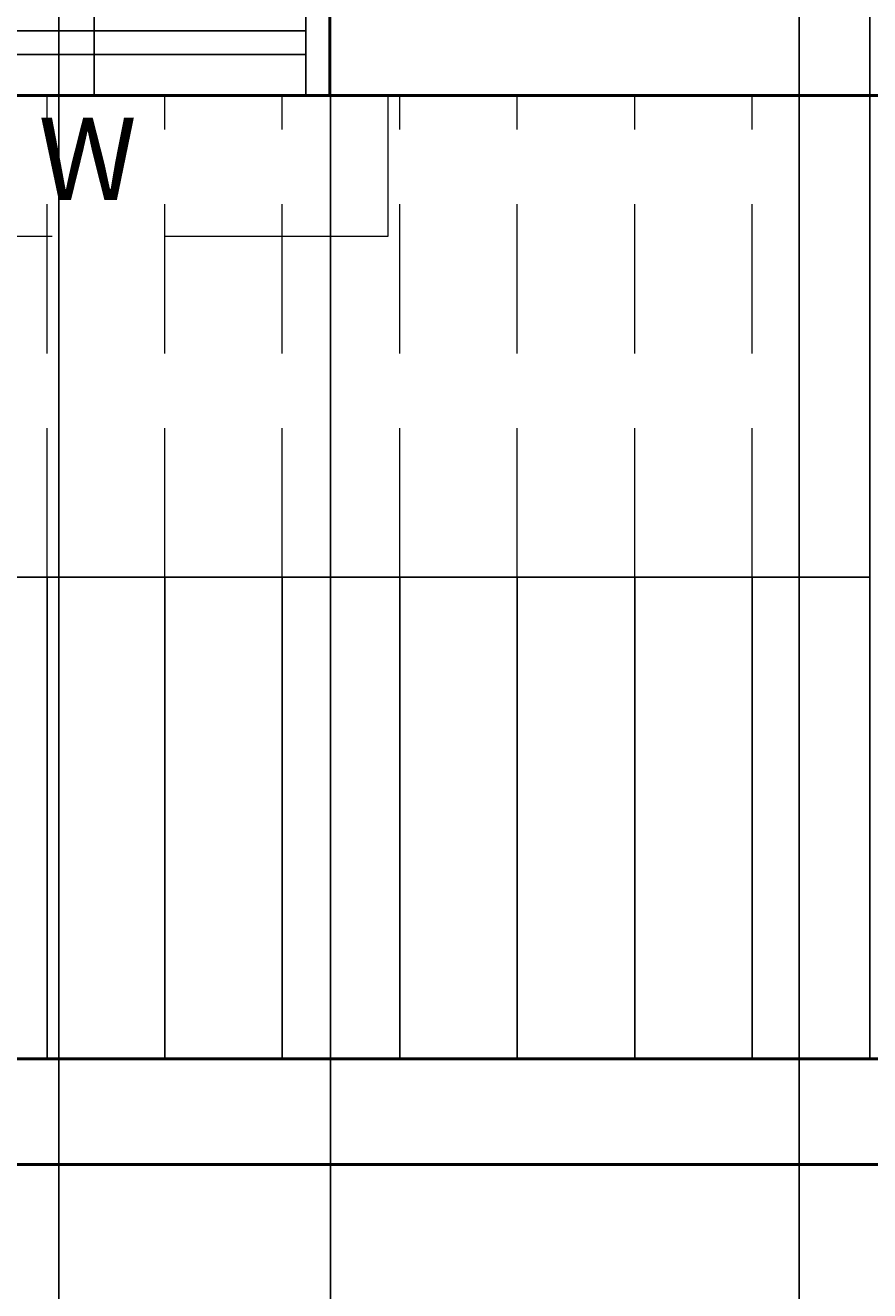
# Model space of a CAD drawing. Units: inches. Extents: x 37 to 824, y -700 to 234.
# Tile 26 of 77: x 224 to 296, y -377 to -269. Entities that reach past the tile are written whole.
import ezdxf

# ---------------------------------------------------------------- set-up
doc = ezdxf.new("R2010")
doc.units = ezdxf.units.IN
doc.header["$MEASUREMENT"] = 0
doc.linetypes.add('DASHED', pattern=[19.05, 12.7, -6.35])
for name, color, linetype, lineweight in [('A-ANNO-DIMS', 2, 'Continuous', 18), ('A-ANNO-TEXT', 7, 'Continuous', 18), ('A-FLOR-STRS', 1, 'Continuous', 25), ('A-FLOR-STRS-OVHD', 1, 'DASHED', 18), ('A-GLAZ', 4, 'Continuous', 25), ('A-ROOF-OVHD', 1, 'DASHED', 18), ('A-WALL', 2, 'Continuous', 50)]:
    doc.layers.add(name, color=color, linetype=linetype, lineweight=lineweight)
doc.styles.get("Standard").update_dxf_attribs({"font": 'arial.ttf'})
doc.dimstyles.get("Standard").update_dxf_attribs({"dimtxt": 0.18, "dimasz": 0.18, "dimexe": 0.18, "dimexo": 0.0625, "dimgap": 0.09, "dimtad": 0, "dimtih": 1, "dimtoh": 1, "dimdec": 1, "dimzin": 0, "dimdsep": 46, "dimlunit": 4, "dimtxsty": 'Standard', "dimcen": 0.09, "dimadec": 0, "dimazin": 0, "dimtfac": 1, "dimtdec": 1, "dimtofl": 0, "dimtmove": 0, "dimatfit": 3, "dimfxl": 1, "dimtolj": 1, "dimtzin": 0, "dimarcsym": 0})

# ---------------------------------------------------------------- blocks, each defined once
blk = doc.blocks.new('WIN-900')
for p, q in [((0, 9), (0, 0)), ((2, 9), (2, 0)), ((20, 9), (20, 0)), ((38, 9), (38, 0)), ((40, 9), (40, 0)), ((38, 5.5), (2, 5.5)), ((38, 3.5), (2, 3.5))]:
    blk.add_line(p, q)
blk = doc.blocks.new('*D77')
at = {"layer": 'A-ANNO-DIMS', "color": 0, "lineweight": -2, "ltscale": 0.5, "transparency": 16777216}
for p, q in [((227.08, 45.5), (227.08, -400.41)), ((290.08, 15.03), (290.08, -400.41)), ((227.26, -400.23), (258.25, -400.23)), ((289.9, -400.23), (258.91, -400.23))]:
    blk.add_line(p, q, dxfattribs=at)
at = {"layer": 'A-ANNO-DIMS', "color": 0, "ltscale": 0.5, "transparency": 16777216}
for points in [[(227.26, -400.2), (227.26, -400.26), (227.08, -400.23)], [(289.9, -400.2), (289.9, -400.26), (290.08, -400.23)]]:
    blk.add_solid(points, dxfattribs=at)
at = {"layer": 'Defpoints', "color": 0, "ltscale": 0.5, "transparency": 16777216}
for p in [(227.08, 45.56), (290.08, 15.09), (290.08, -400.23)]:
    blk.add_point(p, dxfattribs=at)
at = {"layer": 'A-ANNO-DIMS', "color": 0, "ltscale": 0.5, "transparency": 16777216, "insert": (258.58, -400.23), "char_height": 0.18, "attachment_point": 5}
blk.add_mtext('\\A1;5\'-3"', dxfattribs=at)
blk = doc.blocks.new('*D80')
at = {"layer": 'A-ANNO-DIMS', "color": 0, "lineweight": -2, "ltscale": 0.5, "transparency": 16777216}
for p, q in [((170.08, -167.97), (170.08, -400.41)), ((250.19, -167.97), (250.19, -400.41)), ((170.26, -400.23), (209.8, -400.23)), ((250.01, -400.23), (210.46, -400.23))]:
    blk.add_line(p, q, dxfattribs=at)
at = {"layer": 'A-ANNO-DIMS', "color": 0, "ltscale": 0.5, "transparency": 16777216}
for points in [[(170.26, -400.2), (170.26, -400.26), (170.08, -400.23)], [(250.01, -400.2), (250.01, -400.26), (250.19, -400.23)]]:
    blk.add_solid(points, dxfattribs=at)
at = {"layer": 'Defpoints', "color": 0, "ltscale": 0.5, "transparency": 16777216}
for p in [(170.08, -167.91), (250.19, -167.91), (250.19, -400.23)]:
    blk.add_point(p, dxfattribs=at)
at = {"layer": 'A-ANNO-DIMS', "color": 0, "ltscale": 0.5, "transparency": 16777216, "insert": (210.13, -400.23), "char_height": 0.18, "attachment_point": 5}
blk.add_mtext('\\A1;6\'-8"', dxfattribs=at)
blk = doc.blocks.new('*D81')
at = {"layer": 'A-ANNO-DIMS', "color": 0, "lineweight": -2, "ltscale": 0.5, "transparency": 16777216}
for p, q in [((290.08, -164.97), (290.08, -400.41)), ((250.19, -167.97), (250.19, -400.41)), ((250.37, -400.23), (269.8, -400.23)), ((289.9, -400.23), (270.46, -400.23))]:
    blk.add_line(p, q, dxfattribs=at)
at = {"layer": 'A-ANNO-DIMS', "color": 0, "ltscale": 0.5, "transparency": 16777216}
for points in [[(250.37, -400.2), (250.37, -400.26), (250.19, -400.23)], [(289.9, -400.2), (289.9, -400.26), (290.08, -400.23)]]:
    blk.add_solid(points, dxfattribs=at)
at = {"layer": 'Defpoints', "color": 0, "ltscale": 0.5, "transparency": 16777216}
for p in [(290.08, -164.91), (250.19, -167.91), (290.08, -400.23)]:
    blk.add_point(p, dxfattribs=at)
at = {"layer": 'A-ANNO-DIMS', "color": 0, "ltscale": 0.5, "transparency": 16777216, "insert": (270.13, -400.23), "char_height": 0.18, "attachment_point": 5}
blk.add_mtext('\\A1;3\'-4"', dxfattribs=at)
blk = doc.blocks.new('*D87')
at = {"layer": 'A-ANNO-DIMS', "color": 0, "lineweight": -2, "ltscale": 0.5, "transparency": 16777216}
for p, q in [((216.08, -356.85), (216.08, 234.17)), ((216.26, 233.99), (255.75, 233.99)), ((295.9, 233.99), (256.41, 233.99)), ((296.08, -356.85), (296.08, 234.17))]:
    blk.add_line(p, q, dxfattribs=at)
at = {"layer": 'A-ANNO-DIMS', "color": 0, "ltscale": 0.5, "transparency": 16777216}
for points in [[(216.26, 234.02), (216.26, 233.96), (216.08, 233.99)], [(295.9, 234.02), (295.9, 233.96), (296.08, 233.99)]]:
    blk.add_solid(points, dxfattribs=at)
at = {"layer": 'Defpoints', "color": 0, "ltscale": 0.5, "transparency": 16777216}
for p in [(296.08, 233.99), (216.08, -356.91), (296.08, -356.91)]:
    blk.add_point(p, dxfattribs=at)
at = {"layer": 'A-ANNO-DIMS', "color": 0, "ltscale": 0.5, "transparency": 16777216, "insert": (256.08, 233.99), "char_height": 0.18, "attachment_point": 5}
blk.add_mtext('\\A1;6\'-8"', dxfattribs=at)

msp = doc.modelspace()

# ---------------------------------------------------------------- linework, layer by layer
at = {"layer": 'A-FLOR-STRS'}
for p, q in [((170.08, -315.91), (296.08, -315.91)), ((226.08, -315.91), (226.08, -356.91)), ((236.08, -315.91), (236.08, -356.91)), ((246.08, -315.91), (246.08, -356.91)), ((256.08, -315.91), (256.08, -356.91)), ((266.08, -315.91), (266.08, -356.91)), ((276.08, -315.91), (276.08, -356.91)), ((286.08, -315.91), (286.08, -356.91)), ((296.08, -315.91), (296.08, -356.91))]:
    msp.add_line(p, q, dxfattribs=at)
at = {"layer": 'A-FLOR-STRS-OVHD'}
for p, q in [((226.08, -315.91), (226.08, -274.91)), ((236.08, -315.91), (236.08, -274.91)), ((246.08, -315.91), (246.08, -274.91)), ((256.08, -315.91), (256.08, -274.91)), ((266.08, -315.91), (266.08, -274.91)), ((276.08, -315.91), (276.08, -274.91)), ((286.08, -315.91), (286.08, -274.91)), ((296.08, -315.91), (296.08, -274.91))]:
    msp.add_line(p, q, dxfattribs=at)
at = {"layer": 'A-ROOF-OVHD', "ltscale": 1.5}
for p, q in [((250.08, -274.91), (255.08, -274.91)), ((255.08, -274.91), (255.08, -286.91)), ((255.08, -286.91), (205.08, -286.91))]:
    msp.add_line(p, q, dxfattribs=at)
at = {"layer": 'A-WALL'}
for p, q in [((299.08, -274.91), (170.08, -274.91)), ((299.08, -356.91), (170.08, -356.91)), ((428.08, -365.91), (161.08, -365.91))]:
    msp.add_line(p, q, dxfattribs=at)

# ---------------------------------------------------------------- block references
at = {"layer": 'A-GLAZ', "rotation": 180}
msp.add_blockref('WIN-900', (250.08, -265.91), dxfattribs=at)

# ---------------------------------------------------------------- texts
at = {"layer": 'A-ANNO-TEXT'}
msp.add_text('W', height=7, dxfattribs=at).set_placement((225.33, -283.79))

# ---------------------------------------------------------------- dimensions: what is measured, and where the dimension line sits
at = {"layer": 'A-ANNO-DIMS', "ltscale": 0.5}
for base, p1, p2, picture, middle in [((296.08, 233.99), (216.08, -356.91), (296.08, -356.91), '*D87', (256.08, 233.99)), ((290.08, -400.23), (227.08, 45.56), (290.08, 15.09), '*D77', (258.58, -400.23)), ((290.08, -400.23), (250.19, -167.91), (290.08, -164.91), '*D81', (270.13, -400.23)), ((250.19, -400.23), (170.08, -167.91), (250.19, -167.91), '*D80', (210.13, -400.23))]:
    dim = msp.add_linear_dim(base=base, p1=p1, p2=p2, dimstyle='Standard', override={"dimdec": 1, "dimlfac": 1, "dimrnd": 0, "dimzin": 1, "dimdsep": 46, "dimlunit": 4, "dimfrac": 2}, dxfattribs=at)
    dim.commit()
    dim.dimension.update_dxf_attribs({"geometry": picture, "text_midpoint": middle})

doc.saveas('drawing.dxf')
